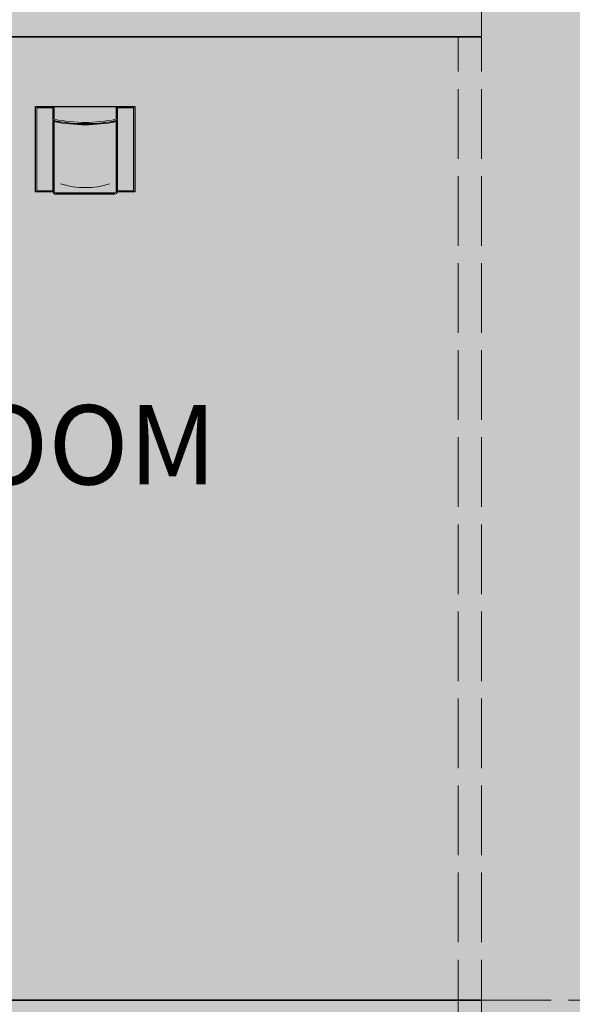
# Model space of a CAD drawing. Units: inches. Extents: x 1704 to 6393, y -157 to 1172.
# Tile 41 of 122: x 2198 to 2293, y 372 to 541. Entities that reach past the tile are written whole.
import ezdxf

# ---------------------------------------------------------------- set-up
doc = ezdxf.new("R2010")
doc.units = ezdxf.units.IN
doc.header["$MEASUREMENT"] = 0
doc.linetypes.add('ACAD_ISO02W100', pattern=[15, 12, -3])
for name, color, linetype, lineweight in [('A-ANNO-DIMS', 7, 'Continuous', 13), ('A-AREA-IDEN', 7, 'Continuous', 18), ('A-FURN', 8, 'Continuous', 18), ('A-WALL-OVHD', 8, 'ACAD_ISO02W100', 13), ('A-WALL-PATT', 7, 'Continuous', 13), ('hachura', 252, 'Continuous', 5), ('moveis', 254, 'Continuous', 5), ('WALLS', 7, 'Continuous', 35)]:
    doc.layers.add(name, color=color, linetype=linetype, lineweight=lineweight)
doc.layers.add('A-FLOR-PATT', color=7, linetype='Continuous', lineweight=13, true_color=0xf2f2f2)
doc.layers.add('MESA', color=7, linetype='Continuous')
doc.styles.get("Standard").update_dxf_attribs({"font": 'arial.ttf'})
doc.dimstyles.get("Standard").update_dxf_attribs({"dimtxt": 6, "dimasz": 2, "dimexe": 0.18, "dimexo": 0.0625, "dimgap": 0.09, "dimtad": 0, "dimtih": 1, "dimtoh": 1, "dimdec": 1, "dimzin": 0, "dimdsep": 46, "dimlunit": 3, "dimtxsty": 'Standard', "dimblk": 'ARCHTICK', "dimcen": 0.09, "dimadec": 0, "dimazin": 0, "dimtfac": 1, "dimtdec": 1, "dimtofl": 0, "dimtmove": 0, "dimatfit": 3, "dimfxl": 1, "dimtolj": 1, "dimtzin": 0, "dimarcsym": 0})

# ---------------------------------------------------------------- blocks, each defined once
blk = doc.blocks.new('Poltrona Palla')
at = {"layer": 'hachura'}
h = blk.add_hatch(color=256, dxfattribs=at)
h.dxf.hatch_style = 1
h.set_gradient(color1=(73, 95, 131), color2=(46, 60, 82), one_color=1, tint=0.25, name='INVCYLINDER')
h.paths.add_polyline_path([(0.265, 0), (-0.265, 0), (-0.265, -0.1089, 0.101458), (0.265, -0.1089)])
h = blk.add_hatch(color=256, dxfattribs=at)
h.dxf.hatch_style = 1
h.set_gradient(color1=(73, 95, 131), color2=(35, 45, 62), one_color=1, tint=0.19)
h.paths.add_polyline_path([(-0.275, -0.01), (-0.415, -0.01), (-0.415, -0.7213), (-0.275, -0.7213)])
h = blk.add_hatch(color=256, dxfattribs=at)
h.dxf.hatch_style = 1
h.set_gradient(color1=(73, 95, 131), color2=(35, 45, 62), one_color=1, tint=0.19)
h.paths.add_polyline_path([(0.415, -0.01), (0.275, -0.01), (0.275, -0.7213), (0.415, -0.7213)])
h = blk.add_hatch(color=256, dxfattribs=at)
h.dxf.hatch_style = 1
h.set_gradient(color1=(73, 95, 131), color2=(35, 45, 62), one_color=1, tint=0.19, name='INVCURVED')
h.paths.add_polyline_path([(0.265, -0.1293, -0.099912), (-0.265, -0.1293), (-0.265, -0.73, 0.414214), (-0.255, -0.74), (0.255, -0.74, 0.414214), (0.265, -0.73)])
at = {"layer": 'MESA'}
for p, q in [((-0.425, 0), (0.425, 0)), ((-0.425, -0.7313), (-0.425, 0)), ((-0.275, -0.73), (-0.275, 0)), ((0.275, 0), (0.275, -0.73)), ((0.425, 0), (0.425, -0.7313)), ((-0.275, -0.7313), (-0.425, -0.7313)), ((0.255, -0.75), (-0.255, -0.75)), ((0.425, -0.7313), (0.275, -0.7313))]:
    blk.add_line(p, q, dxfattribs=at)
for centre, radius, start, end in [((0, 1.1836), 1.3294, 258.06163, 281.93837), ((-0.255, -0.73), 0.02, 180, 270)]:
    blk.add_arc(centre, radius, start, end, dxfattribs=at)
at = {"layer": 'moveis', "ltscale": 0.05}
for p, q in [((-0.265, -0.1089), (-0.265, 0)), ((0.265, 0), (0.265, -0.1089)), ((-0.415, -0.01), (-0.275, -0.01)), ((-0.415, -0.7213), (-0.415, -0.01)), ((0.275, -0.01), (0.415, -0.01)), ((0.415, -0.01), (0.415, -0.7213)), ((-0.265, -0.73), (-0.265, -0.1293)), ((0.265, -0.1293), (0.265, -0.73)), ((-0.275, -0.7213), (-0.415, -0.7213)), ((0.255, -0.74), (-0.255, -0.74)), ((0.415, -0.7213), (0.275, -0.7213))]:
    blk.add_line(p, q, dxfattribs=at)
for centre, radius, start, end in [((0, 1.1836), 1.3194, 258.41345, 281.58655), ((0, 1.1836), 1.3394, 258.5888, 281.4112), ((0, -0.0151), 0.6799, 251.92101, 288.07899), ((-0.255, -0.73), 0.01, 180, 270), ((0.255, -0.73), 0.01, 270, 360), ((0.255, -0.73), 0.02, 270, 360)]:
    blk.add_arc(centre, radius, start, end, dxfattribs=at)
blk = doc.blocks.new('_ArchTick')
at = {"color": 0, "linetype": 'ByBlock', "const_width": 0.15}
blk.add_lwpolyline([(-0.5, -0.5), (0.5, 0.5)], dxfattribs=at)
blk = doc.blocks.new('*D58')
at = {"layer": 'A-ANNO-DIMS', "color": 0, "lineweight": -2, "transparency": 16777216}
for p, q in [((2200.54, 354.32), (2200.54, 357)), ((2200.54, 356.82), (2217.62, 356.82)), ((2217.62, 354.32), (2217.62, 357)), ((2217.62, 356.82), (2219.62, 356.82))]:
    blk.add_line(p, q, dxfattribs=at)
at = {"layer": 'Defpoints', "color": 0, "lineweight": -3, "transparency": 16777216}
for p in [(2217.62, 356.82), (2200.54, 354.26), (2217.62, 354.26)]:
    blk.add_point(p, dxfattribs=at)
at = {"layer": 'A-ANNO-DIMS', "color": 0, "lineweight": -2, "transparency": 16777216, "xscale": 2, "yscale": 2, "zscale": 2, "rotation": 180}
blk.add_blockref('_ArchTick', (2200.54, 356.82), dxfattribs=at)
at = {"layer": 'A-ANNO-DIMS', "color": 0, "lineweight": -2, "transparency": 16777216, "xscale": 2, "yscale": 2, "zscale": 2}
blk.add_blockref('_ArchTick', (2217.62, 356.82), dxfattribs=at)
at = {"layer": 'A-ANNO-DIMS', "color": 0, "transparency": 16777216, "insert": (2262.58, 356.82), "char_height": 6, "attachment_point": 5}
blk.add_mtext('\\A1;PALLA CHAIR 17 TYP.', dxfattribs=at)
blk = doc.blocks.new('*D93')
at = {"layer": 'A-ANNO-DIMS', "color": 0, "lineweight": -2, "transparency": 16777216}
for p, q in [((2605.29, 895.21), (1829.7, 895.21)), ((1829.88, 895.21), (1829.88, 495.87)), ((1829.88, 90.21), (1829.88, 489.56)), ((2605.29, 90.21), (1829.7, 90.21))]:
    blk.add_line(p, q, dxfattribs=at)
at = {"layer": 'Defpoints', "color": 0, "lineweight": -3, "transparency": 16777216}
for p in [(2605.35, 895.21), (1829.88, 90.21), (2605.35, 90.21)]:
    blk.add_point(p, dxfattribs=at)
at = {"layer": 'A-ANNO-DIMS', "color": 0, "lineweight": -2, "transparency": 16777216, "xscale": 2, "yscale": 2, "zscale": 2}
for p, rotation in [((1829.88, 895.21), 90), ((1829.88, 90.21), 270)]:
    blk.add_blockref('_ArchTick', p, dxfattribs=dict(at, rotation=rotation))
at = {"layer": 'A-ANNO-DIMS', "color": 0, "transparency": 16777216, "insert": (1829.88, 492.71), "char_height": 6, "attachment_point": 5}
blk.add_mtext('\\A1;805', dxfattribs=at)

msp = doc.modelspace()

# ---------------------------------------------------------------- hatches: boundary and pattern name
at = {"layer": 'A-FLOR-PATT', "transparency": 33554528}
h = msp.add_hatch(color=256, dxfattribs=at)
h.dxf.hatch_style = 1
h.paths.add_polyline_path([(2325.349, 863.213), (2325.349, 887.213), (2263.349, 887.213), (2167.349, 887.213), (2081.349, 887.213), (2081.349, 719.213), (2277.349, 719.213), (2277.349, 711.213), (2277.349, 372.213), (2349.349, 372.213), (2381.349, 372.213), (2381.349, 364.213), (2353.349, 364.213), (2353.349, 270.213), (2381.349, 270.213), (2381.349, 266.213), (2357.349, 266.213), (2357.349, 98.213), (2381.349, 98.213), (2385.181, 98.213), (2386.482, 98.213), (2424.215, 98.213), (2425.516, 98.213), (2429.349, 98.213), (2597.349, 98.213), (2597.349, 146.213), (2597.349, 218.213), (2597.349, 266.213), (2423.349, 266.213), (2423.349, 270.213), (2473.349, 270.213), (2473.349, 294.213), (2477.349, 294.213), (2477.349, 270.213), (2547.349, 270.213), (2547.349, 364.213), (2477.349, 364.213), (2477.349, 318.213), (2473.349, 318.213), (2473.349, 364.213), (2423.349, 364.213), (2423.349, 372.213), (2469.349, 372.213), (2469.349, 459.213), (2469.349, 538.213), (2350.349, 538.213), (2350.349, 565.713), (2358.349, 565.713), (2358.349, 545.213), (2420.349, 545.213), (2420.349, 610.213), (2358.349, 610.213), (2358.349, 589.713), (2350.349, 589.713), (2350.349, 615.213), (2425.349, 615.213), (2425.349, 607.213), (2425.349, 546.213), (2469.349, 546.213), (2514.349, 546.213), (2514.349, 607.213), (2449.349, 607.213), (2449.349, 615.213), (2451.738, 615.213), (2451.738, 659.213), (2427.738, 659.213), (2427.738, 665.213), (2367.738, 665.213), (2367.738, 667.213), (2367.738, 711.213), (2325.349, 711.213), (2325.349, 719.213), (2325.349, 755.213), (2325.349, 763.213)])
h.paths.add_polyline_path([(2233.858, 822.533, -0.187247), (2233.858, 809.14), (2231.697, 808.804, 0.0848928), (2233.131, 814.486), (2230.424, 814.486, -0.1042581), (2228.553, 808.313), (2217.751, 807.156, -0.2222222), (2217.751, 824.517), (2228.553, 823.359, -0.1042581), (2230.424, 817.186), (2233.131, 817.186, 0.0848928), (2231.697, 822.868)], flags=16)
h.paths.add_polyline_path([(2213.621, 833.197), (2213.621, 798.475), (2156.048, 798.475), (2156.048, 833.197)], flags=16)
h.paths.add_polyline_path([(2203.932, 848.099), (2205.089, 837.296, -0.2222222), (2187.728, 837.296), (2188.885, 848.099, -0.1042581), (2195.058, 849.969), (2195.058, 852.676, 0.0848928), (2189.377, 851.242), (2189.712, 853.404, -0.187247), (2203.105, 853.404), (2203.44, 851.242, 0.0848928), (2197.759, 852.676), (2197.759, 849.969, -0.1042581)], flags=16)
h.paths.add_polyline_path([(2181.941, 837.296, -0.2222222), (2164.58, 837.296), (2165.737, 848.099, -0.1042581), (2171.91, 849.969), (2171.91, 852.676, 0.0848928), (2166.229, 851.242), (2166.564, 853.404, -0.187247), (2179.957, 853.404), (2180.292, 851.242, 0.0848928), (2174.611, 852.676), (2174.611, 849.969, -0.1042581), (2180.784, 848.099)], flags=16)
h.paths.add_polyline_path([(2205.089, 794.376), (2203.932, 783.574, -0.1042581), (2197.759, 781.703), (2197.759, 778.996, 0.0848928), (2203.44, 780.43), (2203.105, 778.269, -0.187247), (2189.712, 778.269), (2189.377, 780.43, 0.0848928), (2195.058, 778.996), (2195.058, 781.703, -0.1042581), (2188.885, 783.574), (2187.728, 794.376, -0.2222222)], flags=16)
h.paths.add_polyline_path([(2181.941, 794.376), (2180.784, 783.574, -0.1042581), (2174.611, 781.703), (2174.611, 778.996, 0.0848928), (2180.292, 780.43), (2179.957, 778.269, -0.187247), (2166.564, 778.269), (2166.229, 780.43, 0.0848928), (2171.91, 778.996), (2171.91, 781.703, -0.1042581), (2165.737, 783.574), (2164.58, 794.376, -0.2222222)], flags=16)
h.paths.add_polyline_path([(2151.918, 807.156), (2141.116, 808.313, -0.1042581), (2139.245, 814.486), (2136.539, 814.486, 0.0848928), (2137.972, 808.804), (2135.811, 809.14, -0.187247), (2135.811, 822.533), (2137.972, 822.868, 0.0848928), (2136.539, 817.186), (2139.245, 817.186, -0.1042581), (2141.116, 823.359), (2151.918, 824.517, -0.2222222)], flags=16)
h.paths.add_polyline_path([(2357.868, 363.41), (2358.814, 363.41, 0.7537605)], flags=16)
h.paths.add_polyline_path([(2372.241, 363.117), (2372.248, 363.117), (2372.248, 363.343), (2371.302, 363.343), (2371.302, 363.139, -1.3603913)], flags=16)
h.paths.add_polyline_path([(2371.309, 272.716), (2371.302, 272.716), (2371.302, 272.49), (2372.248, 272.49), (2372.248, 272.693, -1.3603913)], flags=16)
h.paths.add_polyline_path([(2357.875, 272.716), (2357.868, 272.716), (2357.868, 272.49), (2358.814, 272.49), (2358.814, 272.693, -1.3603913)], flags=16)
h.paths.add_polyline_path([(2353.769, 363.074), (2376.347, 363.074), (2376.347, 272.759), (2353.769, 272.759)], flags=16)
h.paths.add_polyline_path([(2354.772, 362.07), (2375.344, 362.07), (2375.344, 273.762), (2354.772, 273.762)], flags=0)
h.paths.add_polyline_path([(2357.868, 363.343), (2358.814, 363.343), (2358.814, 363.117), (2357.868, 363.117)], flags=16)
h.paths.add_polyline_path([(2359.288, 359.184), (2359.288, 360.063), (2370.828, 360.063), (2370.828, 359.184), (2374.332, 359.184), (2374.332, 358.464), (2372.835, 358.464), (2372.835, 357.541), (2374.332, 357.541), (2374.332, 356.82), (2372.835, 356.82), (2372.835, 355.898), (2374.332, 355.898), (2374.332, 355.177), (2372.835, 355.177), (2372.835, 354.254), (2374.332, 354.254), (2374.332, 353.534), (2372.835, 353.534), (2372.835, 352.611), (2374.332, 352.611), (2374.332, 351.89), (2372.835, 351.89), (2372.835, 350.968), (2374.332, 350.968), (2374.332, 350.247), (2372.835, 350.247), (2372.835, 349.324), (2374.332, 349.324), (2374.332, 348.604), (2372.835, 348.604), (2372.835, 347.681), (2374.332, 347.681), (2374.332, 346.96), (2372.835, 346.96), (2372.835, 346.038), (2374.332, 346.038), (2374.332, 345.317), (2372.835, 345.317), (2372.835, 344.395), (2374.332, 344.395), (2374.332, 343.674), (2372.835, 343.674), (2372.835, 342.751), (2374.332, 342.751), (2374.332, 342.03), (2372.835, 342.03), (2372.835, 341.108), (2374.332, 341.108), (2374.332, 340.387), (2372.835, 340.387), (2372.835, 339.465), (2374.332, 339.465), (2374.332, 338.744), (2372.835, 338.744), (2372.835, 337.821), (2374.332, 337.821), (2374.332, 337.1), (2372.835, 337.1), (2372.835, 336.178), (2374.332, 336.178), (2374.332, 335.457), (2372.835, 335.457), (2372.835, 334.535), (2374.332, 334.535), (2374.332, 333.814), (2372.835, 333.814), (2372.835, 332.891), (2374.332, 332.891), (2374.332, 332.171), (2372.835, 332.171), (2372.835, 331.248), (2374.332, 331.248), (2374.332, 330.527), (2372.835, 330.527), (2372.835, 329.605), (2374.332, 329.605), (2374.332, 328.884), (2372.835, 328.884), (2372.835, 327.961), (2374.332, 327.961), (2374.332, 327.241), (2372.835, 327.241), (2372.835, 326.318), (2374.332, 326.318), (2374.332, 325.597), (2372.835, 325.597), (2372.835, 324.675), (2374.332, 324.675), (2374.332, 323.954), (2372.835, 323.954), (2372.835, 323.031), (2374.332, 323.031), (2374.332, 322.311), (2372.835, 322.311), (2372.835, 321.388), (2374.332, 321.388), (2374.332, 320.667), (2372.835, 320.667), (2372.835, 319.745), (2374.332, 319.745), (2374.332, 319.024), (2372.835, 319.024), (2372.835, 318.102), (2374.332, 318.102), (2374.332, 317.381), (2372.835, 317.381), (2372.835, 316.458), (2374.332, 316.458), (2374.332, 315.737), (2372.835, 315.737), (2372.835, 314.815), (2374.332, 314.815), (2374.332, 314.094), (2372.835, 314.094), (2372.835, 313.172), (2374.332, 313.172), (2374.332, 312.451), (2372.835, 312.451), (2372.835, 311.528), (2374.332, 311.528), (2374.332, 310.807), (2372.835, 310.807), (2372.835, 309.885), (2374.332, 309.885), (2374.332, 309.164), (2372.835, 309.164), (2372.835, 308.242), (2374.332, 308.242), (2374.332, 307.521), (2372.835, 307.521), (2372.835, 306.598), (2374.332, 306.598), (2374.332, 305.878), (2372.835, 305.878), (2372.835, 304.955), (2374.332, 304.955), (2374.332, 304.234), (2372.835, 304.234), (2372.835, 303.312), (2374.332, 303.312), (2374.332, 302.591), (2372.835, 302.591), (2372.835, 301.668), (2374.332, 301.668), (2374.332, 300.948), (2372.835, 300.948), (2372.835, 300.025), (2374.332, 300.025), (2374.332, 299.304), (2372.835, 299.304), (2372.835, 298.382), (2374.332, 298.382), (2374.332, 297.661), (2372.835, 297.661), (2372.835, 296.738), (2374.332, 296.738), (2374.332, 296.018), (2372.835, 296.018), (2372.835, 295.095), (2374.332, 295.095), (2374.332, 294.374), (2372.835, 294.374), (2372.835, 293.452), (2374.332, 293.452), (2374.332, 292.731), (2372.835, 292.731), (2372.835, 291.809), (2374.332, 291.809), (2374.332, 291.088), (2372.835, 291.088), (2372.835, 290.165), (2374.332, 290.165), (2374.332, 289.444), (2372.835, 289.444), (2372.835, 288.522), (2374.332, 288.522), (2374.332, 287.801), (2372.835, 287.801), (2372.835, 286.879), (2374.332, 286.879), (2374.332, 286.158), (2372.835, 286.158), (2372.835, 285.235), (2374.332, 285.235), (2374.332, 284.514), (2372.835, 284.514), (2372.835, 283.592), (2374.332, 283.592), (2374.332, 282.871), (2372.835, 282.871), (2372.835, 281.949), (2374.332, 281.949), (2374.332, 281.228), (2372.835, 281.228), (2372.835, 280.305), (2374.332, 280.305), (2374.332, 279.585), (2372.835, 279.585), (2372.835, 278.662), (2374.332, 278.662), (2374.332, 277.941), (2372.835, 277.941), (2372.835, 277.019), (2374.332, 277.019), (2374.332, 276.298), (2370.828, 276.298), (2370.828, 275.769), (2359.288, 275.769), (2359.288, 276.298), (2355.784, 276.298), (2355.784, 277.019), (2357.281, 277.019), (2357.281, 277.941), (2355.784, 277.941), (2355.784, 278.662), (2357.281, 278.662), (2357.281, 279.585), (2355.784, 279.585), (2355.784, 280.305), (2357.281, 280.305), (2357.281, 281.228), (2355.784, 281.228), (2355.784, 281.949), (2357.281, 281.949), (2357.281, 282.871), (2355.784, 282.871), (2355.784, 283.592), (2357.281, 283.592), (2357.281, 284.514), (2355.784, 284.514), (2355.784, 285.235), (2357.281, 285.235), (2357.281, 286.158), (2355.784, 286.158), (2355.784, 286.879), (2357.281, 286.879), (2357.281, 287.801), (2355.784, 287.801), (2355.784, 288.522), (2357.281, 288.522), (2357.281, 289.444), (2355.784, 289.444), (2355.784, 290.165), (2357.281, 290.165), (2357.281, 291.088), (2355.784, 291.088), (2355.784, 291.809), (2357.281, 291.809), (2357.281, 292.731), (2355.784, 292.731), (2355.784, 293.452), (2357.281, 293.452), (2357.281, 294.374), (2355.784, 294.374), (2355.784, 295.095), (2357.281, 295.095), (2357.281, 296.018), (2355.784, 296.018), (2355.784, 296.738), (2357.281, 296.738), (2357.281, 297.661), (2355.784, 297.661), (2355.784, 298.382), (2357.281, 298.382), (2357.281, 299.304), (2355.784, 299.304), (2355.784, 300.025), (2357.281, 300.025), (2357.281, 300.948), (2355.784, 300.948), (2355.784, 301.668), (2357.281, 301.668), (2357.281, 302.591), (2355.784, 302.591), (2355.784, 303.312), (2357.281, 303.312), (2357.281, 304.234), (2355.784, 304.234), (2355.784, 304.955), (2357.281, 304.955), (2357.281, 305.878), (2355.784, 305.878), (2355.784, 306.598), (2357.281, 306.598), (2357.281, 307.521), (2355.784, 307.521), (2355.784, 308.242), (2357.281, 308.242), (2357.281, 309.164), (2355.784, 309.164), (2355.784, 309.885), (2357.281, 309.885), (2357.281, 310.807), (2355.784, 310.807), (2355.784, 311.528), (2357.281, 311.528), (2357.281, 312.451), (2355.784, 312.451), (2355.784, 313.172), (2357.281, 313.172), (2357.281, 314.094), (2355.784, 314.094), (2355.784, 314.815), (2357.281, 314.815), (2357.281, 315.737), (2355.784, 315.737), (2355.784, 316.458), (2357.281, 316.458), (2357.281, 317.381), (2355.784, 317.381), (2355.784, 318.102), (2357.281, 318.102), (2357.281, 319.024), (2355.784, 319.024), (2355.784, 319.745), (2357.281, 319.745), (2357.281, 320.667), (2355.784, 320.667), (2355.784, 321.388), (2357.281, 321.388), (2357.281, 322.311), (2355.784, 322.311), (2355.784, 323.031), (2357.281, 323.031), (2357.281, 323.954), (2355.784, 323.954), (2355.784, 324.675), (2357.281, 324.675), (2357.281, 325.597), (2355.784, 325.597), (2355.784, 326.318), (2357.281, 326.318), (2357.281, 327.241), (2355.784, 327.241), (2355.784, 327.961), (2357.281, 327.961), (2357.281, 328.884), (2355.784, 328.884), (2355.784, 329.605), (2357.281, 329.605), (2357.281, 330.527), (2355.784, 330.527), (2355.784, 331.248), (2357.281, 331.248), (2357.281, 332.171), (2355.784, 332.171), (2355.784, 332.891), (2357.281, 332.891), (2357.281, 333.814), (2355.784, 333.814), (2355.784, 334.535), (2357.281, 334.535), (2357.281, 335.457), (2355.784, 335.457), (2355.784, 336.178), (2357.281, 336.178), (2357.281, 337.1), (2355.784, 337.1), (2355.784, 337.821), (2357.281, 337.821), (2357.281, 338.744), (2355.784, 338.744), (2355.784, 339.465), (2357.281, 339.465), (2357.281, 340.387), (2355.784, 340.387), (2355.784, 341.108), (2357.281, 341.108), (2357.281, 342.03), (2355.784, 342.03), (2355.784, 342.751), (2357.281, 342.751), (2357.281, 343.674), (2355.784, 343.674), (2355.784, 344.395), (2357.281, 344.395), (2357.281, 345.317), (2355.784, 345.317), (2355.784, 346.038), (2357.281, 346.038), (2357.281, 346.96), (2355.784, 346.96), (2355.784, 347.681), (2357.281, 347.681), (2357.281, 348.604), (2355.784, 348.604), (2355.784, 349.324), (2357.281, 349.324), (2357.281, 350.247), (2355.784, 350.247), (2355.784, 350.968), (2357.281, 350.968), (2357.281, 351.89), (2355.784, 351.89), (2355.784, 352.611), (2357.281, 352.611), (2357.281, 353.534), (2355.784, 353.534), (2355.784, 354.254), (2357.281, 354.254), (2357.281, 355.177), (2355.784, 355.177), (2355.784, 355.898), (2357.281, 355.898), (2357.281, 356.82), (2355.784, 356.82), (2355.784, 357.541), (2357.281, 357.541), (2357.281, 358.464), (2355.784, 358.464), (2355.784, 359.184)], flags=0)
h = msp.add_hatch(color=256, dxfattribs=at)
h.dxf.hatch_style = 1
h.paths.add_polyline_path([(2273.349, 538.213), (2081.349, 538.213), (2081.349, 372.213), (2273.349, 372.213)])
h.paths.add_polyline_path([(2189.542, 505.951), (2184.316, 505.951), (2184.316, 505.591), (2169.442, 505.591), (2169.442, 505.951), (2164.216, 505.951, -0.4142136), (2163.814, 506.353), (2163.814, 526.093, -0.4142136), (2164.216, 526.495), (2189.542, 526.495, -0.4142136), (2189.944, 526.093), (2189.944, 506.353, -0.4142136)], flags=16)
h.paths.add_polyline_path([(2200.535, 511.491), (2200.535, 526.191), (2217.621, 526.191), (2217.621, 511.491), (2214.605, 511.491, -0.3946213), (2214.203, 511.116), (2203.952, 511.116, -0.3946213), (2203.551, 511.491)], flags=16)
h.paths.add_polyline_path([(2200.736, 511.692), (2200.736, 525.99), (2203.55, 525.99), (2203.55, 523.838, 0.1045605), (2214.605, 523.838), (2214.605, 525.99), (2217.42, 525.99), (2217.42, 511.692), (2214.605, 511.692), (2214.605, 523.838, -0.1045605), (2203.55, 523.838), (2203.55, 511.692)], flags=0)
h.paths.add_polyline_path([(2203.952, 511.317, -0.4142136), (2203.751, 511.518), (2203.751, 523.591, 0.099912), (2214.404, 523.591), (2214.404, 511.518, -0.4142136), (2214.203, 511.317)], flags=0)
h.paths.add_polyline_path([(2184.084, 516.015, -0.0686795), (2169.674, 516.015), (2169.674, 522.073), (2184.084, 522.073)], flags=0)
h.paths.add_polyline_path([(2183.325, 518.606, -0.0772766), (2170.433, 518.606), (2170.433, 521.123, -0.0235462), (2183.325, 521.123)], flags=0)
h.paths.add_polyline_path([(2135.029, 507.225, -0.1405189), (2135.191, 507.834, -0.0513838), (2135.029, 507.797)], flags=16)
h.paths.add_polyline_path([(2146.318, 498.997, -0.0311848), (2144.279, 499.202, -0.1719602), (2141.865, 499.263, -0.2234326), (2139.482, 499.263, -0.1719602), (2137.068, 499.202, -0.0311848), (2135.029, 498.997, -0.066975), (2135.029, 505.313, -0.0276914), (2136.841, 505.144), (2136.841, 506.777), (2136.576, 506.777), (2136.576, 507.371, 0.039911), (2145.741, 507.448, 0.2546956), (2146.318, 507.225), (2146.318, 507.269, 0.1305786), (2146.156, 507.834, -0.0704067), (2145.953, 507.935, -0.011584), (2145.714, 508.002, -0.2546956), (2145.137, 507.779, -0.2546956), (2145.361, 508.355, -0.0259693), (2145.107, 516.407, -0.0070422), (2144.025, 516.297, -0.1828112), (2142.939, 516.218, -0.2042746), (2142.015, 516.175, -0.1805419), (2139.348, 516.174, -0.0000184), (2139.345, 516.174, -0.2035615), (2138.425, 516.217, -0.0000237), (2138.421, 516.217, -0.1818152), (2137.34, 516.296, -0.0071635), (2136.24, 516.407, 0.007166), (2136.162, 518.63, 0.314303), (2135.854, 518.974, -0.1253469), (2135.537, 518.935, -0.2546956), (2135.76, 519.512, -0.0162662), (2135.67, 519.849, -0.296972), (2135.535, 520.8, -0.227702), (2135.464, 521.698, 0.1283977), (2132.757, 521.718), (2132.757, 525.785, -0.4142136), (2133.331, 526.359), (2148.015, 526.359, -0.4142136), (2148.589, 525.785), (2148.589, 521.718, -0.0118936), (2148.835, 521.65, -0.2546956), (2149.412, 521.873, -0.2546956), (2149.188, 521.296, -0.0417628), (2149.188, 508.355, -0.2546956), (2149.412, 507.779, -0.2546956), (2148.835, 508.002, -0.011584), (2148.596, 507.935, -0.2124435), (2147.949, 507.813, -0.2363999), (2147.423, 507.772, -0.3143526), (2147.126, 507.772, -0.2363999), (2146.6, 507.813, -0.0879275), (2146.318, 507.797), (2146.318, 507.225, -0.2546956), (2145.741, 507.448, -0.0042329), (2144.771, 507.371), (2144.771, 506.777), (2144.506, 506.777), (2144.506, 505.144, -0.0276914), (2146.318, 505.313, -0.066975)], flags=16)
h.paths.add_polyline_path([(2141.865, 505.047, 0.2234326), (2139.482, 505.047, 0.1738145), (2137.043, 505.1), (2137.043, 506.317), (2137.335, 506.317), (2137.335, 505.184, -0.1522072), (2139.482, 505.047, -0.2234326), (2141.865, 505.047, -0.1522072), (2144.011, 505.184), (2144.011, 506.317), (2144.304, 506.317), (2144.304, 505.1, 0.1738145)], flags=0)
h.paths.add_polyline_path([(2145.233, 522.986, 0.0079197), (2144.017, 523.111, 0.1826165), (2142.931, 523.19, 0.2042746), (2142.008, 523.233, 0.1806536), (2139.339, 523.233, 0.2042746), (2138.415, 523.19, 0.1826165), (2137.33, 523.111, 0.0079197), (2136.114, 522.986, 0.1967082), (2135.679, 523.212, 0.047677), (2135.755, 524.004), (2134.638, 521.852), (2134.376, 524.691, -0.2583282), (2135.029, 526.359, -0.0890464), (2135.632, 525.01, -0.1830277), (2145.715, 525.01, -0.0890464), (2146.318, 526.359, -0.2583282), (2146.971, 524.691), (2146.709, 521.852), (2145.592, 524.004, 0.047677), (2145.668, 523.212, 0.1967082)], flags=0)
h.paths.add_polyline_path([(2144.419, 519.027, -0.0368796), (2136.927, 519.027, -0.0368796)], flags=0)
h.paths.add_polyline_path([(2273.349, 629.213), (2213.349, 629.213), (2213.349, 573.213), (2213.349, 545.213), (2273.349, 545.213)])
h.paths.add_polyline_path([(2273.349, 711.213), (2207.349, 711.213), (2207.349, 709.213), (2231.349, 709.213), (2231.349, 707.213), (2207.349, 707.213), (2207.349, 631.213), (2273.349, 631.213)])
h.paths.add_polyline_path([(2273.349, 364.213), (2081.349, 364.213), (2081.349, 202.213), (2225.349, 202.213), (2229.181, 202.213), (2230.482, 202.213), (2268.215, 202.213), (2269.516, 202.213), (2273.349, 202.213)])
h.paths.add_polyline_path([(2203.551, 339.558, 0.3946213), (2203.952, 339.183), (2214.203, 339.183), (2214.203, 339.384), (2203.751, 339.384), (2203.751, 339.558)], flags=16)
h.paths.add_polyline_path([(2203.55, 351.7), (2203.55, 339.759), (2200.535, 339.759), (2200.535, 354.258), (2217.621, 354.258), (2217.621, 339.558), (2214.404, 339.558), (2214.404, 351.659, -0.101837)], flags=16)
h.paths.add_polyline_path([(2214.404, 354.057), (2214.605, 354.057), (2214.605, 354.258), (2214.404, 354.258)], flags=16)
h.paths.add_polyline_path([(2189.542, 334.018), (2184.316, 334.018), (2184.316, 333.658), (2169.442, 333.658), (2169.442, 334.018), (2164.216, 334.018, -0.4142136), (2163.814, 334.42), (2163.814, 354.161, -0.4142136), (2164.216, 354.563), (2189.542, 354.563, -0.4142136), (2189.944, 354.161), (2189.944, 334.42, -0.4142136)], flags=16)
h.paths.add_polyline_path([(2184.084, 344.083, -0.0686795), (2169.674, 344.083), (2169.674, 349.85), (2165.7, 350.14), (2188.058, 350.14), (2184.084, 349.85)], flags=0)
h.paths.add_polyline_path([(2183.325, 346.673, -0.0772766), (2170.433, 346.673), (2170.433, 349.19, -0.0235462), (2183.325, 349.19)], flags=0)
h.paths.add_polyline_path([(2134.638, 349.919), (2134.376, 352.758, -0.2583282), (2135.029, 354.426), (2133.331, 354.426, 0.4142136), (2132.757, 353.852), (2132.757, 349.785, -0.0886664)], flags=16)
h.paths.add_polyline_path([(2136.114, 351.053, -0.0079197), (2137.33, 351.178, -0.1826165), (2138.415, 351.257, -0.2042746), (2139.339, 351.3, -0.1806536), (2142.008, 351.3, -0.2042746), (2142.931, 351.257, -0.1826165), (2144.017, 351.178, -0.0079197), (2145.233, 351.053, -0.1967082), (2145.668, 351.279, -0.047677), (2145.592, 352.071, 0.1133241), (2135.755, 352.071, -0.047677), (2135.679, 351.279, -0.1967082)], flags=16)
h.paths.add_polyline_path([(2145.184, 346.697, 0.0331414), (2145.361, 336.423, 0.2546956), (2145.137, 335.846, 0.3030408), (2145.781, 336.164, 0.2903634), (2146.6, 335.88, 0.2363999), (2147.126, 335.839, -0.280712), (2147.275, 336.69, -0.280712), (2147.423, 335.839, 0.2363999), (2147.949, 335.88, 0.2903634), (2148.768, 336.164, 0.3030408), (2149.412, 335.846, 0.2546956), (2149.188, 336.423, 0.0417628), (2149.188, 349.363, 0.2546956), (2149.412, 349.94, 0.2546956), (2148.835, 349.717, 0.1405058), (2145.883, 349.765, -0.227702), (2145.812, 348.867, -0.296972), (2145.677, 347.916, -0.0162662), (2145.586, 347.579, -0.2546956), (2145.81, 347.002, -0.1253469), (2145.493, 347.041, 0.314303)], flags=16)
h.paths.add_polyline_path([(2135.029, 335.292, -0.1405189), (2135.191, 335.901, -0.1399435), (2134.747, 335.88, -0.2363999), (2134.22, 335.839, -0.3143526), (2133.924, 335.839, -0.280712), (2134.072, 336.69, -0.280712), (2134.22, 335.839, 0.2363999), (2134.747, 335.88, 0.2903634), (2135.566, 336.164, 0.3030408), (2136.209, 335.846, 0.2546956), (2135.985, 336.423, 0.0331414), (2136.162, 346.697, 0.314303), (2135.854, 347.041, -0.1253469), (2135.537, 347.002, -0.2546956), (2135.76, 347.579, -0.0162662), (2135.67, 347.916, -0.296972), (2135.535, 348.867, -0.2999866), (2135.599, 350.01, -0.0330719), (2135.76, 350.7, -0.3502076), (2135.604, 351.492), (2134.638, 349.919), (2135.604, 351.492, 0.3502076), (2135.76, 350.7, 0.0330719), (2135.599, 350.01, 0.2999866), (2135.535, 348.867, 0.296972), (2135.67, 347.916, 0.0279375), (2135.971, 347.698, 0.3576436), (2135.537, 347.002, 0.1253469), (2135.854, 347.041, -0.3555912), (2136.165, 346.637, -0.0329482), (2135.985, 336.423, -0.2546956), (2136.209, 335.846, -0.2546956), (2135.632, 336.069, -0.011584), (2135.393, 336.003, -0.1222327), (2135.029, 335.864)], flags=16)
h.paths.add_polyline_path([(2136.841, 335.42), (2136.783, 335.423), (2136.783, 334.844), (2136.841, 334.471)], flags=16)
h.paths.add_polyline_path([(2146.318, 327.064, -0.0311848), (2144.279, 327.269, -0.1719602), (2141.865, 327.33, -0.2234326), (2139.482, 327.33, -0.1719602), (2137.068, 327.269, -0.0311848), (2135.029, 327.064, -0.066975), (2135.029, 333.38, -0.0311848), (2137.068, 333.175, -0.1719602), (2139.482, 333.114, -0.2234326), (2141.865, 333.114, -0.1522072), (2144.011, 333.251), (2144.011, 334.384), (2144.304, 335.406, 0.0020345), (2144.771, 335.438), (2144.771, 334.844), (2144.506, 333.211, -0.0276914), (2146.318, 333.38, -0.066975)], flags=16)
h.paths.add_polyline_path([(2137.129, 334.384), (2137.335, 334.384), (2137.335, 333.251), (2137.129, 333.195)], flags=16)
h.paths.add_polyline_path([(2144.419, 347.094, -0.0368796), (2136.927, 347.094, -0.0368796)], flags=16)
h = msp.add_hatch(color=256, dxfattribs=at)
h.dxf.hatch_style = 1
h.paths.add_polyline_path([(2349.349, 372.213), (2277.349, 372.213), (2277.349, 364.213), (2349.349, 364.213)])
h.paths.add_polyline_path([(2277.349, 372.213), (2273.349, 372.213), (2273.349, 364.213), (2277.349, 364.213)])
h.paths.add_polyline_path([(2277.349, 364.213), (2273.349, 364.213), (2273.349, 202.213), (2277.349, 202.213)])
h.paths.add_polyline_path([(2277.349, 538.213), (2273.349, 538.213), (2273.349, 372.213), (2277.349, 372.213)])
h.paths.add_polyline_path([(2277.349, 629.213), (2273.349, 629.213), (2273.349, 545.213), (2277.349, 545.213)])
h.paths.add_polyline_path([(2277.349, 711.213), (2273.349, 711.213), (2273.349, 631.213), (2277.349, 631.213)])
h.paths.add_polyline_path([(2277.349, 631.213), (2273.349, 631.213), (2273.349, 629.213), (2277.349, 629.213)])
at = {"layer": 'A-WALL-PATT', "transparency": 33554643}
h = msp.add_hatch(color=256, dxfattribs=at)
h.dxf.hatch_style = 1
h.paths.add_polyline_path([(2167.349, 895.213), (2073.349, 895.213), (2073.349, 887.213), (2081.349, 887.213), (2167.349, 887.213)])
h.paths.add_polyline_path([(2465.349, 895.213), (2273.349, 895.213), (2273.349, 903.213), (2263.349, 903.213), (2263.349, 895.213), (2263.349, 887.213), (2325.349, 887.213), (2325.349, 863.213), (2333.349, 863.213), (2333.349, 887.213), (2465.349, 887.213)])
h.paths.add_polyline_path([(2533.349, 895.213), (2513.349, 895.213), (2513.349, 887.213), (2513.349, 861.213), (2517.349, 861.213), (2517.349, 887.213), (2533.349, 887.213)])
h.paths.add_polyline_path([(2605.349, 895.213), (2581.349, 895.213), (2581.349, 887.213), (2597.349, 887.213), (2597.349, 854.213), (2605.349, 854.213)])
h.paths.add_polyline_path([(2605.349, 752.213), (2629.349, 752.213), (2629.349, 716.213), (2605.349, 716.213), (2605.349, 712.213), (2719.349, 712.213), (2719.349, 716.213), (2631.349, 716.213), (2631.349, 754.213), (2605.349, 754.213), (2605.349, 794.213), (2597.349, 794.213), (2597.349, 787.213), (2517.349, 787.213), (2517.349, 813.213), (2513.349, 813.213), (2513.349, 783.213), (2517.349, 783.213), (2597.349, 783.213), (2597.349, 719.213), (2517.349, 719.213), (2517.349, 753.213), (2513.349, 753.213), (2513.349, 719.213), (2365.349, 719.213), (2365.349, 763.213), (2325.349, 763.213), (2325.349, 755.213), (2357.349, 755.213), (2357.349, 719.213), (2325.349, 719.213), (2325.349, 711.213), (2547.349, 711.213), (2547.349, 615.213), (2449.349, 615.213), (2449.349, 607.213), (2514.349, 607.213), (2514.349, 546.213), (2439.349, 546.213), (2425.349, 546.213), (2425.349, 607.213), (2425.349, 615.213), (2350.349, 615.213), (2350.349, 589.713), (2358.349, 589.713), (2358.349, 610.213), (2420.349, 610.213), (2420.349, 545.213), (2358.349, 545.213), (2358.349, 565.713), (2350.349, 565.713), (2350.349, 538.213), (2469.349, 538.213), (2469.349, 459.213), (2469.349, 372.213), (2423.349, 372.213), (2423.349, 364.213), (2473.349, 364.213), (2473.349, 318.213), (2477.349, 318.213), (2477.349, 364.213), (2547.349, 364.213), (2547.349, 352.213), (2549.349, 352.213), (2549.349, 364.213), (2597.349, 364.213), (2597.349, 328.213), (2549.349, 328.213), (2547.349, 328.213), (2547.349, 326.213), (2549.349, 326.213), (2597.349, 326.213), (2605.349, 326.213), (2605.349, 377.057), (2597.349, 377.057), (2597.349, 372.213), (2477.349, 372.213), (2477.349, 451.213), (2597.349, 451.213), (2605.349, 451.213), (2605.349, 459.213), (2597.349, 459.213), (2477.349, 459.213), (2477.349, 538.213), (2597.349, 538.213), (2597.349, 495.213), (2605.349, 495.213), (2605.349, 512.213), (2631.349, 512.213), (2631.349, 568.213), (2605.349, 568.213), (2605.349, 577.213), (2597.349, 577.213), (2597.349, 542.213), (2518.349, 542.213), (2518.349, 607.213), (2532.349, 607.213), (2605.349, 607.213), (2605.349, 615.213), (2597.349, 615.213), (2551.349, 615.213), (2551.349, 711.213), (2597.349, 711.213), (2597.349, 645.213), (2605.349, 645.213), (2605.349, 712.213), (2605.349, 716.213)])
h.paths.add_polyline_path([(2605.349, 566.213), (2629.349, 566.213), (2629.349, 514.213), (2605.349, 514.213)], flags=16)
h.paths.add_polyline_path([(2381.349, 372.213), (2349.349, 372.213), (2349.349, 202.213), (2337.349, 202.213), (2337.349, 194.213), (2349.349, 194.213), (2349.349, 90.213), (2349.349, 72.213), (2357.349, 72.213), (2357.349, 90.213), (2381.349, 90.213), (2381.349, 98.213), (2357.349, 98.213), (2357.349, 266.213), (2381.349, 266.213), (2381.349, 270.213), (2353.349, 270.213), (2353.349, 364.213), (2381.349, 364.213)])
h.paths.add_polyline_path([(2605.349, 302.213), (2597.349, 302.213), (2597.349, 270.213), (2477.349, 270.213), (2477.349, 294.213), (2473.349, 294.213), (2473.349, 270.213), (2423.349, 270.213), (2423.349, 266.213), (2597.349, 266.213), (2597.349, 218.213), (2605.349, 218.213)])
h.paths.add_polyline_path([(2605.349, 146.213), (2597.349, 146.213), (2597.349, 98.213), (2429.349, 98.213), (2429.349, 90.213), (2597.349, 90.213), (2597.349, 72.213), (2605.349, 72.213), (2605.349, 90.213)])
h.paths.add_polyline_path([(2225.349, 202.213), (2049.349, 202.213), (2049.349, 194.213), (2225.349, 194.213)])
h.paths.add_polyline_path([(2289.349, 202.213), (2277.349, 202.213), (2273.349, 202.213), (2269.516, 202.213), (2269.516, 194.213), (2273.349, 194.213), (2277.349, 194.213), (2289.349, 194.213)])
h.paths.add_polyline_path([(2273.349, 372.213), (2029.19, 372.213), (2029.19, 364.213), (2273.349, 364.213)])
h.paths.add_polyline_path([(2277.349, 545.213), (2213.349, 545.213), (2213.349, 573.213), (2205.349, 573.213), (2177.349, 573.213), (2177.349, 545.213), (2073.349, 545.213), (2073.349, 538.213), (2081.349, 538.213), (2277.349, 538.213)])
h.paths.add_polyline_path([(2181.349, 545.213), (2181.349, 569.213), (2205.349, 569.213), (2205.349, 545.213)], flags=16)
h.paths.add_polyline_path([(2277.349, 719.213), (2081.349, 719.213), (2073.349, 719.213), (2073.349, 711.213), (2154.575, 711.213), (2205.349, 711.213), (2205.349, 687.213), (2205.349, 629.213), (2213.349, 629.213), (2273.349, 629.213), (2273.349, 631.213), (2207.349, 631.213), (2207.349, 707.213), (2231.349, 707.213), (2231.349, 709.213), (2207.349, 709.213), (2207.349, 711.213), (2277.349, 711.213)])

# ---------------------------------------------------------------- linework, layer by layer
at = {"layer": 'A-WALL-OVHD'}
for p, q in [((2277.349, 202.213), (2277.349, 711.213)), ((2273.349, 202.213), (2273.349, 538.213)), ((2277.349, 372.213), (2349.349, 372.213))]:
    msp.add_line(p, q, dxfattribs=at)
at = {"layer": 'WALLS'}
for p, q in [((2277.349, 538.213), (2081.349, 538.213)), ((2277.349, 372.213), (2029.19, 372.213))]:
    msp.add_line(p, q, dxfattribs=at)

# ---------------------------------------------------------------- block references
at = {"layer": 'A-FURN', "xscale": 20.10025524054769, "yscale": 20.10025524054769, "zscale": 20.10025524054769}
msp.add_blockref('Poltrona Palla', (2209.078, 526.191), dxfattribs=at)

# ---------------------------------------------------------------- texts
at = {"layer": 'A-AREA-IDEN'}
msp.add_text('DINING ROOM', height=13.6672, dxfattribs=at).set_placement((2109.317, 461.082))

# ---------------------------------------------------------------- dimensions: what is measured, and where the dimension line sits
at = {"layer": 'A-ANNO-DIMS'}
dim = msp.add_linear_dim(base=(1829.878, 90.213), p1=(2605.349, 895.213), p2=(2605.349, 90.213), angle=90, dimstyle='Standard', override={"dimdec": 0, "dimlfac": 1, "dimrnd": 0, "dimzin": 0, "dimdsep": 46, "dimlunit": 2}, dxfattribs=at)
dim.commit()
dim.dimension.update_dxf_attribs({"geometry": '*D93', "text_midpoint": (1829.878, 492.713)})
dim = msp.add_linear_dim(base=(2217.621, 356.821), p1=(2200.535, 354.258), p2=(2217.621, 354.258), text='PALLA CHAIR <> TYP.', dimstyle='Standard', override={"dimdec": 0, "dimlfac": 1, "dimrnd": 0, "dimzin": 0, "dimdsep": 46, "dimlunit": 2}, dxfattribs=at)
dim.commit()
dim.dimension.update_dxf_attribs({"geometry": '*D58', "text_midpoint": (2262.58, 356.821)})

doc.saveas('drawing.dxf')
